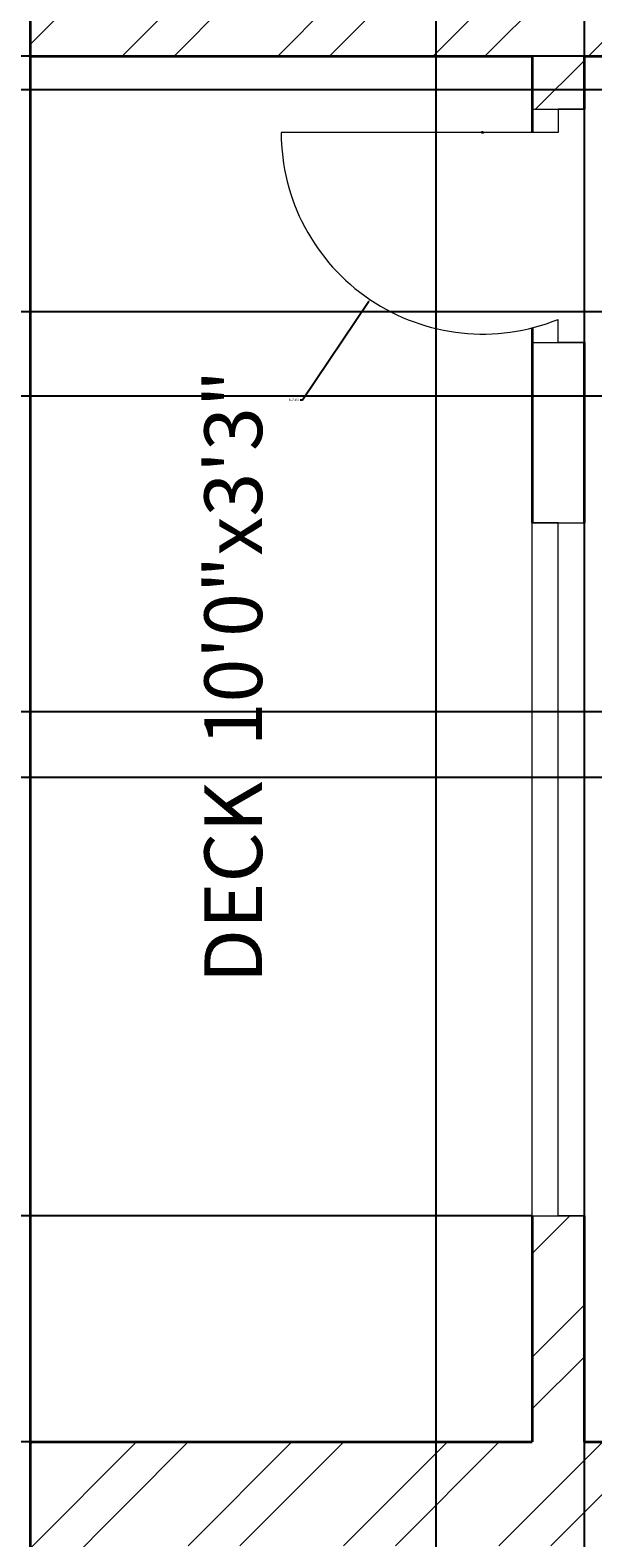
# Model space of a CAD drawing. Units: inches. Extents: x 1748 to 2382, y 1346 to 2284.
# Tile 18 of 26: x 1822 to 1871, y 1971 to 2102. Entities that reach past the tile are written whole.
import ezdxf

# ---------------------------------------------------------------- set-up
doc = ezdxf.new("R2010")
doc.units = ezdxf.units.IN
for name, color, linetype, lineweight in [('A-ANNO-DIMS', 2, 'Continuous', 18), ('A-AREA-IDEN', 7, 'Continuous', 18), ('A-DOOR', 21, 'Continuous', 18), ('A-GLAZ', 191, 'Continuous', 18), ('A-WALL', 7, 'Continuous', 35), ('A-WALL-PATT', 9, 'Continuous', 13)]:
    doc.layers.add(name, color=color, linetype=linetype, lineweight=lineweight)
doc.styles.get("Standard").update_dxf_attribs({"font": 'arial.ttf'})
doc.dimstyles.get("Standard").update_dxf_attribs({"dimtxt": 0.18, "dimasz": 0.18, "dimexe": 0.18, "dimexo": 0.0625, "dimgap": 0.09, "dimtad": 0, "dimtih": 1, "dimtoh": 1, "dimdec": 4, "dimzin": 0, "dimdsep": 46, "dimtxsty": 'Standard', "dimcen": 0.09, "dimadec": 0, "dimazin": 0, "dimtfac": 1, "dimtdec": 4, "dimtofl": 0, "dimtmove": 0, "dimatfit": 3, "dimfxl": 1, "dimtolj": 1, "dimtzin": 0, "dimarcsym": 0})

# ---------------------------------------------------------------- blocks, each defined once
blk = doc.blocks.new('WIN-60-SHALLOW')
for p, q in [((0, 60), (4.5, 60)), ((0, 60), (0, 0)), ((4.5, 60), (2.25, 60)), ((2.25, 60), (2.25, 0)), ((4.5, 60), (4.5, 0)), ((2.25, 0), (0, 0)), ((0, 0), (4.5, 0))]:
    blk.add_line(p, q)
blk = doc.blocks.new('*D41')
at = {"layer": 'A-ANNO-DIMS', "color": 0, "lineweight": -2, "transparency": 16777216}
for p, q in [((1821.96, 1854.91), (1821.96, 2274.93)), ((1822.14, 2274.75), (1839.16, 2274.75)), ((1856.96, 2274.75), (1839.95, 2274.75)), ((1857.14, 1854.91), (1857.14, 2274.93))]:
    blk.add_line(p, q, dxfattribs=at)
at = {"layer": 'A-ANNO-DIMS', "color": 0, "transparency": 16777216}
for points in [[(1822.14, 2274.78), (1822.14, 2274.72), (1821.96, 2274.75)], [(1856.96, 2274.78), (1856.96, 2274.72), (1857.14, 2274.75)]]:
    blk.add_solid(points, dxfattribs=at)
at = {"layer": 'Defpoints', "color": 0, "transparency": 16777216}
for p in [(1857.14, 2274.75), (1821.96, 1854.85), (1857.14, 1854.85)]:
    blk.add_point(p, dxfattribs=at)
at = {"layer": 'A-ANNO-DIMS', "color": 0, "transparency": 16777216, "insert": (1839.55, 2274.75), "char_height": 0.18, "attachment_point": 5}
blk.add_mtext('\\A1;35.18', dxfattribs=at)
blk = doc.blocks.new('*D45')
at = {"layer": 'A-ANNO-DIMS', "color": 0, "lineweight": -2, "transparency": 16777216}
for p, q in [((1821.9, 2232.85), (1779.88, 2232.85)), ((1780.06, 2232.67), (1780.06, 2116.07)), ((1780.06, 1999.11), (1780.06, 2115.71)), ((1865.4, 1998.93), (1779.88, 1998.93))]:
    blk.add_line(p, q, dxfattribs=at)
at = {"layer": 'A-ANNO-DIMS', "color": 0, "transparency": 16777216}
for points in [[(1780.03, 2232.67), (1780.09, 2232.67), (1780.06, 2232.85)], [(1780.03, 1999.11), (1780.09, 1999.11), (1780.06, 1998.93)]]:
    blk.add_solid(points, dxfattribs=at)
at = {"layer": 'Defpoints', "color": 0, "transparency": 16777216}
for p in [(1780.06, 2232.85), (1821.96, 2232.85), (1865.46, 1998.93)]:
    blk.add_point(p, dxfattribs=at)
at = {"layer": 'A-ANNO-DIMS', "color": 0, "transparency": 16777216, "insert": (1780.06, 2115.89), "char_height": 0.18, "attachment_point": 5}
blk.add_mtext('\\A1;233.9', dxfattribs=at)
blk = doc.blocks.new('*D50')
at = {"layer": 'A-ANNO-DIMS', "color": 0, "lineweight": -2, "transparency": 16777216}
for p, q in [((1869.96, 2223.79), (1869.96, 1360.47)), ((1908.44, 2223.79), (1908.44, 1360.47)), ((1870.14, 1360.65), (1888.81, 1360.65)), ((1908.26, 1360.65), (1889.6, 1360.65))]:
    blk.add_line(p, q, dxfattribs=at)
at = {"layer": 'A-ANNO-DIMS', "color": 0, "transparency": 16777216}
for points in [[(1870.14, 1360.68), (1870.14, 1360.62), (1869.96, 1360.65)], [(1908.26, 1360.68), (1908.26, 1360.62), (1908.44, 1360.65)]]:
    blk.add_solid(points, dxfattribs=at)
at = {"layer": 'Defpoints', "color": 0, "transparency": 16777216}
for p in [(1869.96, 2223.85), (1908.44, 2223.85), (1908.44, 1360.65)]:
    blk.add_point(p, dxfattribs=at)
at = {"layer": 'A-ANNO-DIMS', "color": 0, "transparency": 16777216, "insert": (1889.2, 1360.65), "char_height": 0.18, "attachment_point": 5}
blk.add_mtext('\\A1;38.48', dxfattribs=at)
blk = doc.blocks.new('*D57')
at = {"layer": 'A-ANNO-DIMS', "color": 0, "lineweight": -2, "transparency": 16777216}
for p, q in [((2288.4, 2099.35), (1779.88, 2099.35)), ((1780.06, 2099.17), (1780.06, 2088.46)), ((1780.06, 2077.38), (1780.06, 2088.09)), ((2288.4, 2077.2), (1779.88, 2077.2))]:
    blk.add_line(p, q, dxfattribs=at)
at = {"layer": 'A-ANNO-DIMS', "color": 0, "transparency": 16777216}
for points in [[(1780.03, 2099.17), (1780.09, 2099.17), (1780.06, 2099.35)], [(1780.03, 2077.38), (1780.09, 2077.38), (1780.06, 2077.2)]]:
    blk.add_solid(points, dxfattribs=at)
at = {"layer": 'Defpoints', "color": 0, "transparency": 16777216}
for p in [(1780.06, 2099.35), (2288.46, 2099.35), (2288.46, 2077.2)]:
    blk.add_point(p, dxfattribs=at)
at = {"layer": 'A-ANNO-DIMS', "color": 0, "transparency": 16777216, "insert": (1780.06, 2088.28), "char_height": 0.18, "attachment_point": 5}
blk.add_mtext('\\A1;22.15', dxfattribs=at)
blk = doc.blocks.new('*D63')
at = {"layer": 'A-ANNO-DIMS', "color": 0, "lineweight": -2, "transparency": 16777216}
for p, q in [((2253.72, 2042.57), (1779.88, 2042.57)), ((1780.06, 2042.39), (1780.06, 2039.92)), ((1780.06, 2037.08), (1780.06, 2039.55)), ((2253.72, 2036.9), (1779.88, 2036.9))]:
    blk.add_line(p, q, dxfattribs=at)
at = {"layer": 'A-ANNO-DIMS', "color": 0, "transparency": 16777216}
for points in [[(1780.03, 2042.39), (1780.09, 2042.39), (1780.06, 2042.57)], [(1780.03, 2037.08), (1780.09, 2037.08), (1780.06, 2036.9)]]:
    blk.add_solid(points, dxfattribs=at)
at = {"layer": 'Defpoints', "color": 0, "transparency": 16777216}
for p in [(1780.06, 2042.57), (2253.78, 2042.57), (2253.78, 2036.9)]:
    blk.add_point(p, dxfattribs=at)
at = {"layer": 'A-ANNO-DIMS', "color": 0, "transparency": 16777216, "insert": (1780.06, 2039.74), "char_height": 0.18, "attachment_point": 5}
blk.add_mtext('\\A1;5.673', dxfattribs=at)
blk = doc.blocks.new('*D69')
at = {"layer": 'A-ANNO-DIMS', "color": 0, "lineweight": -2, "transparency": 16777216}
for p, q in [((1865.4, 1998.93), (1779.88, 1998.93)), ((1780.06, 1998.75), (1780.06, 1989.32)), ((1780.06, 1979.53), (1780.06, 1988.96)), ((1821.9, 1979.35), (1779.88, 1979.35))]:
    blk.add_line(p, q, dxfattribs=at)
at = {"layer": 'A-ANNO-DIMS', "color": 0, "transparency": 16777216}
for points in [[(1780.03, 1998.75), (1780.09, 1998.75), (1780.06, 1998.93)], [(1780.03, 1979.53), (1780.09, 1979.53), (1780.06, 1979.35)]]:
    blk.add_solid(points, dxfattribs=at)
at = {"layer": 'Defpoints', "color": 0, "transparency": 16777216}
for p in [(1780.06, 1998.93), (1865.46, 1998.93), (1821.96, 1979.35)]:
    blk.add_point(p, dxfattribs=at)
at = {"layer": 'A-ANNO-DIMS', "color": 0, "transparency": 16777216, "insert": (1780.06, 1989.14), "char_height": 0.18, "attachment_point": 5}
blk.add_mtext('\\A1;19.58', dxfattribs=at)
blk = doc.blocks.new('*D76')
at = {"layer": 'A-ANNO-DIMS', "color": 0, "lineweight": -2, "transparency": 16777216}
for p, q in [((2025.9, 2096.43), (1779.88, 2096.43)), ((1780.06, 2096.25), (1780.06, 2083.35)), ((1780.06, 2070.08), (1780.06, 2082.98)), ((2025.9, 2069.9), (1779.88, 2069.9))]:
    blk.add_line(p, q, dxfattribs=at)
at = {"layer": 'A-ANNO-DIMS', "color": 0, "transparency": 16777216}
for points in [[(1780.03, 2096.25), (1780.09, 2096.25), (1780.06, 2096.43)], [(1780.03, 2070.08), (1780.09, 2070.08), (1780.06, 2069.9)]]:
    blk.add_solid(points, dxfattribs=at)
at = {"layer": 'Defpoints', "color": 0, "transparency": 16777216}
for p in [(1780.06, 2096.43), (2025.96, 2096.43), (2025.96, 2069.9)]:
    blk.add_point(p, dxfattribs=at)
at = {"layer": 'A-ANNO-DIMS', "color": 0, "transparency": 16777216, "insert": (1780.06, 2083.16), "char_height": 0.18, "attachment_point": 5}
blk.add_mtext('\\A1;26.535', dxfattribs=at)
blk = doc.blocks.new('*D94')
at = {"layer": 'A-ANNO-DIMS', "color": 0, "lineweight": -2, "transparency": 16777216}
for p, q in [((1861.17, 2092.66), (1861.17, 2092.84)), ((1861.08, 2092.75), (1861.26, 2092.75)), ((1845.55, 2069.59), (1851.31, 2078.13)), ((1845.37, 2069.59), (1845.55, 2069.59))]:
    blk.add_line(p, q, dxfattribs=at)
at = {"layer": 'A-ANNO-DIMS', "color": 0, "transparency": 16777216}
blk.add_solid([(1851.28, 2078.14), (1851.33, 2078.11), (1851.41, 2078.27)], dxfattribs=at)
at = {"layer": 'Defpoints', "color": 0, "transparency": 16777216}
for p in [(1861.17, 2092.75), (1851.41, 2078.27)]:
    blk.add_point(p, dxfattribs=at)
at = {"layer": 'A-ANNO-DIMS', "color": 0, "transparency": 16777216, "insert": (1844.82, 2069.59), "char_height": 0.18, "attachment_point": 5}
blk.add_mtext('\\A1;R17.464', dxfattribs=at)

msp = doc.modelspace()

# ---------------------------------------------------------------- hatches: boundary and pattern name
at = {"layer": 'A-WALL-PATT'}
h = msp.add_hatch(dxfattribs=at)
h.set_pattern_fill('ANSI32', color=256)
h.paths.add_polyline_path([(1908.4445, 2232.8497), (1821.9607, 2232.8497), (1821.9607, 2223.8497), (1865.4607, 2223.8497), (1865.4607, 2209.9185), (1869.9607, 2209.9185), (1869.9607, 2223.8497), (1908.4445, 2223.8497), (1908.4445, 2228.3497)])
h.paths.add_polyline_path([(2040.0683, 2232.8497), (1968.4445, 2232.8497), (1968.4445, 2223.8497), (2025.9607, 2223.8497), (2025.9607, 2130.3497), (2032.1341, 2130.3497), (2032.1341, 2132.5997), (2032.1341, 2134.8497), (2030.4607, 2134.8497), (2030.4607, 2223.8497), (2040.0683, 2223.8497)])
h.paths.add_polyline_path([(2091.3969, 2232.8497), (2064.0683, 2232.8497), (2064.0683, 2223.8497), (2078.4607, 2223.8497), (2078.4607, 2134.8497), (2051.1563, 2134.8497), (2051.1563, 2130.3497), (2078.4607, 2130.3497), (2078.4607, 2128.6813), (2082.9607, 2128.6813), (2082.9607, 2130.3497), (2086.1879, 2130.3497), (2086.1879, 2132.5997), (2086.1879, 2134.8497), (2082.9607, 2134.8497), (2082.9607, 2223.8497), (2091.3969, 2223.8497), (2091.3969, 2228.3497)])
h.paths.add_polyline_path([(2167.0164, 2232.8497), (2115.3969, 2232.8497), (2115.3969, 2223.8497), (2130.9607, 2223.8497), (2130.9607, 2134.8497), (2106.9607, 2134.8497), (2106.9607, 2130.3497), (2135.4607, 2130.3497), (2135.4607, 2223.8497), (2167.0164, 2223.8497), (2167.0164, 2228.3497)])
h.paths.add_polyline_path([(1869.9607, 2149.9185), (1865.4607, 2149.9185), (1865.4607, 2127.8942), (1869.9607, 2127.8942)])
h.paths.add_polyline_path([(2082.9607, 2104.4871), (2080.7107, 2104.4871), (2078.4607, 2104.4871), (2078.4607, 2103.8497), (1869.9607, 2103.8497), (1869.9607, 2108.6062), (1867.7107, 2108.6062), (1865.4607, 2108.6062), (1865.4607, 2103.8497), (1821.9607, 2103.8497), (1821.9607, 2099.3497), (1865.4607, 2099.3497), (1865.4607, 2094.7509), (1869.9607, 2094.7509), (1869.9607, 2099.3497), (2025.9607, 2099.3497), (2025.9607, 2096.4326), (2030.4607, 2096.4326), (2030.4607, 2099.3497), (2082.9607, 2099.3497)])
h.paths.add_polyline_path([(1928.9457, 1401.1212), (2176.8693, 1401.1212), (2176.8693, 1438.214), (1928.9457, 1438.214)], flags=9)
h.paths.add_polyline_path([(2122.2668, 2048.1927), (2177.9387, 2048.1927), (2177.9387, 2066.85), (2122.2668, 2066.85)], flags=9)
h.paths.add_polyline_path([(2272.688, 2153.8197), (2272.688, 2216.746), (2262.3845, 2216.746), (2262.3845, 2153.8197)], flags=9)
h.paths.add_polyline_path([(2157.2928, 2166.5593), (2196.3822, 2166.5593), (2196.3822, 2185.2167), (2157.2928, 2185.2167)], flags=9)
h.paths.add_polyline_path([(2089.3407, 2162.0698), (2124.3987, 2162.0698), (2124.3987, 2180.7272), (2089.3407, 2180.7272)], flags=9)
h.paths.add_polyline_path([(2037.4521, 2160.0913), (2072.5101, 2160.0913), (2072.5101, 2178.7486), (2037.4521, 2178.7486)], flags=9)
h.paths.add_polyline_path([(1884.7894, 2104.1554), (1923.6297, 2104.1554), (1923.6297, 2122.8127), (1884.7894, 2122.8127)], flags=9)
h.paths.add_polyline_path([(1851.2832, 2142.9749), (1851.2832, 2199.3051), (1840.9796, 2199.3051), (1840.9796, 2142.9749)], flags=9)
h.paths.add_polyline_path([(1844.8763, 2017.2834), (1844.8763, 2073.6136), (1834.5728, 2073.6136), (1834.5728, 2017.2834)], flags=9)
h.paths.add_polyline_path([(1897.1577, 2073.1279), (1935.9981, 2073.1279), (1935.9981, 2091.7853), (1897.1577, 2091.7853)], flags=9)
h.paths.add_polyline_path([(1952.3395, 1802.4231), (2008.0114, 1802.4231), (2008.0114, 1821.0805), (1952.3395, 1821.0805)], flags=9)
h.paths.add_polyline_path([(1978.8184, 1857.6841), (2017.7338, 1857.6841), (2017.7338, 1876.3415), (1978.8184, 1876.3415)], flags=9)
h.paths.add_polyline_path([(1979.6513, 1925.9516), (2008.8089, 1925.9516), (2008.8089, 1944.6089), (1979.6513, 1944.6089)], flags=9)
h.paths.add_polyline_path([(1838.5553, 1860.3527), (1877.3957, 1860.3527), (1877.3957, 1879.01), (1838.5553, 1879.01)], flags=9)
h.paths.add_polyline_path([(1883.9018, 1787.3013), (1883.9018, 1843.6315), (1873.5983, 1843.6315), (1873.5983, 1787.3013)], flags=9)
h.paths.add_polyline_path([(1873.7079, 1509.1938), (1873.7079, 1583.7709), (1863.4044, 1583.7709), (1863.4044, 1509.1938)], flags=9)
h.paths.add_polyline_path([(1916.2259, 1603.3681), (1955.0663, 1603.3681), (1955.0663, 1622.0254), (1916.2259, 1622.0254)], flags=9)
h.paths.add_polyline_path([(1876.3013, 1636.757), (1876.3013, 1693.0871), (1865.9978, 1693.0871), (1865.9978, 1636.757)], flags=9)
h.paths.add_polyline_path([(1921.3138, 1521.8316), (1964.0662, 1521.8316), (1964.0662, 1540.489), (1921.3138, 1540.489)], flags=9)
h.paths.add_polyline_path([(2017.5657, 1497.5078), (2046.7983, 1497.5078), (2046.7983, 1516.1651), (2017.5657, 1516.1651)], flags=9)
h.paths.add_polyline_path([(2066.8661, 1499.3902), (2096.0988, 1499.3902), (2096.0988, 1518.0475), (2066.8661, 1518.0475)], flags=9)
h.paths.add_polyline_path([(2155.4835, 1571.6596), (2198.2358, 1571.6596), (2198.2358, 1590.3169), (2155.4835, 1590.3169)], flags=9)
h.paths.add_polyline_path([(2094.9136, 1664.6812), (2150.5855, 1664.6812), (2150.5855, 1683.3386), (2094.9136, 1683.3386)], flags=9)
h.paths.add_polyline_path([(2257.6902, 1863.1628), (2269.8935, 1863.1628), (2269.8935, 1873.4664), (2257.6902, 1873.4664)], flags=9)
h.paths.add_polyline_path([(2164.0748, 1880.3089), (2189.8694, 1880.3089), (2189.8694, 1890.6124), (2164.0748, 1890.6124)], flags=9)
h.paths.add_polyline_path([(2239.4394, 1931.0585), (2268.8187, 1931.0585), (2268.8187, 1949.7159), (2239.4394, 1949.7159)], flags=9)
h = msp.add_hatch(dxfattribs=at)
h.set_pattern_fill('ANSI32', color=256)
h.paths.add_polyline_path([(2297.4607, 2232.8497), (2203.0164, 2232.8497), (2203.0164, 2223.8497), (2244.9607, 2223.8497), (2244.9607, 2127.8554), (2249.4607, 2127.8554), (2249.4607, 2223.8497), (2297.4607, 2223.8497)])
h.paths.add_polyline_path([(2297.4607, 2103.8497), (2249.4607, 2103.8497), (2249.4607, 2106.7497), (2247.2107, 2106.7497), (2244.9607, 2106.7497), (2244.9607, 2103.8497), (2130.9607, 2103.8497), (2130.9607, 2099.3497), (2288.4607, 2099.3497), (2288.4607, 2077.2008), (2297.4607, 2077.2008)])
h.paths.add_polyline_path([(1928.9457, 1401.1212), (2176.8693, 1401.1212), (2176.8693, 1438.214), (1928.9457, 1438.214)], flags=9)
h.paths.add_polyline_path([(2122.2668, 2048.1927), (2177.9387, 2048.1927), (2177.9387, 2066.85), (2122.2668, 2066.85)], flags=9)
h.paths.add_polyline_path([(2272.688, 2153.8197), (2272.688, 2216.746), (2262.3845, 2216.746), (2262.3845, 2153.8197)], flags=25)
h.paths.add_polyline_path([(2157.2928, 2166.5593), (2196.3822, 2166.5593), (2196.3822, 2185.2167), (2157.2928, 2185.2167)], flags=9)
h.paths.add_polyline_path([(2089.3407, 2162.0698), (2124.3987, 2162.0698), (2124.3987, 2180.7272), (2089.3407, 2180.7272)], flags=9)
h.paths.add_polyline_path([(2037.4521, 2160.0913), (2072.5101, 2160.0913), (2072.5101, 2178.7486), (2037.4521, 2178.7486)], flags=9)
h.paths.add_polyline_path([(1884.7894, 2104.1554), (1923.6297, 2104.1554), (1923.6297, 2122.8127), (1884.7894, 2122.8127)], flags=9)
h.paths.add_polyline_path([(1851.2832, 2142.9749), (1851.2832, 2199.3051), (1840.9796, 2199.3051), (1840.9796, 2142.9749)], flags=9)
h.paths.add_polyline_path([(1844.8763, 2017.2834), (1844.8763, 2073.6136), (1834.5728, 2073.6136), (1834.5728, 2017.2834)], flags=9)
h.paths.add_polyline_path([(1897.1577, 2073.1279), (1935.9981, 2073.1279), (1935.9981, 2091.7853), (1897.1577, 2091.7853)], flags=9)
h.paths.add_polyline_path([(1952.3395, 1802.4231), (2008.0114, 1802.4231), (2008.0114, 1821.0805), (1952.3395, 1821.0805)], flags=9)
h.paths.add_polyline_path([(1978.8184, 1857.6841), (2017.7338, 1857.6841), (2017.7338, 1876.3415), (1978.8184, 1876.3415)], flags=9)
h.paths.add_polyline_path([(1979.6513, 1925.9516), (2008.8089, 1925.9516), (2008.8089, 1944.6089), (1979.6513, 1944.6089)], flags=9)
h.paths.add_polyline_path([(1838.5553, 1860.3527), (1877.3957, 1860.3527), (1877.3957, 1879.01), (1838.5553, 1879.01)], flags=9)
h.paths.add_polyline_path([(1883.9018, 1787.3013), (1883.9018, 1843.6315), (1873.5983, 1843.6315), (1873.5983, 1787.3013)], flags=9)
h.paths.add_polyline_path([(1873.7079, 1509.1938), (1873.7079, 1583.7709), (1863.4044, 1583.7709), (1863.4044, 1509.1938)], flags=9)
h.paths.add_polyline_path([(1916.2259, 1603.3681), (1955.0663, 1603.3681), (1955.0663, 1622.0254), (1916.2259, 1622.0254)], flags=9)
h.paths.add_polyline_path([(1876.3013, 1636.757), (1876.3013, 1693.0871), (1865.9978, 1693.0871), (1865.9978, 1636.757)], flags=9)
h.paths.add_polyline_path([(1921.3138, 1521.8316), (1964.0662, 1521.8316), (1964.0662, 1540.489), (1921.3138, 1540.489)], flags=9)
h.paths.add_polyline_path([(2017.5657, 1497.5078), (2046.7983, 1497.5078), (2046.7983, 1516.1651), (2017.5657, 1516.1651)], flags=9)
h.paths.add_polyline_path([(2066.8661, 1499.3902), (2096.0988, 1499.3902), (2096.0988, 1518.0475), (2066.8661, 1518.0475)], flags=9)
h.paths.add_polyline_path([(2155.4835, 1571.6596), (2198.2358, 1571.6596), (2198.2358, 1590.3169), (2155.4835, 1590.3169)], flags=9)
h.paths.add_polyline_path([(2094.9136, 1664.6812), (2150.5855, 1664.6812), (2150.5855, 1683.3386), (2094.9136, 1683.3386)], flags=9)
h.paths.add_polyline_path([(2257.6902, 1863.1628), (2269.8935, 1863.1628), (2269.8935, 1873.4664), (2257.6902, 1873.4664)], flags=9)
h.paths.add_polyline_path([(2164.0748, 1880.3089), (2189.8694, 1880.3089), (2189.8694, 1890.6124), (2164.0748, 1890.6124)], flags=9)
h.paths.add_polyline_path([(2239.4394, 1931.0585), (2268.8187, 1931.0585), (2268.8187, 1949.7159), (2239.4394, 1949.7159)], flags=9)
h = msp.add_hatch(dxfattribs=at)
h.set_pattern_fill('ANSI32', color=256)
h.paths.add_polyline_path([(1919.6777, 1476.8497), (1900.6426, 1476.8497), (1900.6426, 1522.0826), (1898.3926, 1522.0826), (1896.1426, 1522.0826), (1896.1426, 1476.8497), (1857.1426, 1476.8497), (1857.1426, 1467.8497), (1896.1426, 1467.8497), (1919.6777, 1467.8497), (1919.6777, 1472.3497)])
h.paths.add_polyline_path([(2018.7873, 1472.3497), (2018.7873, 1476.8497), (2010.9607, 1476.8497), (2010.9607, 1560.8497), (2034.9607, 1560.8497), (2034.9607, 1565.3497), (2006.4607, 1565.3497), (2006.4607, 1476.8497), (1955.6777, 1476.8497), (1955.6777, 1467.8497), (2018.7873, 1467.8497)])
h.paths.add_polyline_path([(2152.3354, 1472.3497), (2152.3354, 1476.8497), (2115.9607, 1476.8497), (2115.9607, 1565.3497), (2109.2204, 1565.3497), (2109.2204, 1563.0997), (2109.2204, 1560.8497), (2111.4607, 1560.8497), (2111.4607, 1476.8497), (2095.3617, 1476.8497), (2095.3617, 1467.8497), (2152.3354, 1467.8497)])
h.paths.add_polyline_path([(2071.3617, 1476.8497), (2063.4607, 1476.8497), (2063.4607, 1560.8497), (2090.1865, 1560.8497), (2090.1865, 1565.3497), (2063.4607, 1565.3497), (2063.4607, 1572.5485), (2061.2107, 1572.5485), (2058.9607, 1572.5485), (2058.9607, 1565.3497), (2055.6281, 1565.3497), (2055.6281, 1560.8497), (2058.9607, 1560.8497), (2058.9607, 1476.8497), (2042.7873, 1476.8497), (2042.7873, 1467.8497), (2071.3617, 1467.8497), (2071.3617, 1472.3497)])
h.paths.add_polyline_path([(2297.4607, 1506.5652), (2288.4607, 1506.5652), (2288.4607, 1476.8497), (2212.3354, 1476.8497), (2212.3354, 1467.8497), (2297.4607, 1467.8497)])
h.paths.add_polyline_path([(2297.4607, 1645.3038), (2288.4607, 1645.3038), (2288.4607, 1605.8497), (2058.9607, 1605.8497), (2058.9607, 1600.1857), (2061.2107, 1600.1857), (2063.4607, 1600.1857), (2063.4607, 1601.3497), (2288.4607, 1601.3497), (2288.4607, 1566.5652), (2297.4607, 1566.5652)])
h.paths.add_polyline_path([(2010.9607, 1609.0561), (2008.7107, 1609.0561), (2006.4607, 1609.0561), (2006.4607, 1605.8497), (1900.6426, 1605.8497), (1900.6426, 1609.7171), (1898.3926, 1609.7171), (1896.1426, 1609.7171), (1896.1426, 1605.8497), (1857.1426, 1605.8497), (1857.1426, 1601.3497), (1896.1426, 1601.3497), (1896.1426, 1542.5447), (1900.6426, 1542.5447), (1900.6426, 1601.3497), (2010.9607, 1601.3497)])
h.paths.add_polyline_path([(1928.9457, 1401.1212), (2176.8693, 1401.1212), (2176.8693, 1438.214), (1928.9457, 1438.214)], flags=9)
h.paths.add_polyline_path([(2122.2668, 2048.1927), (2177.9387, 2048.1927), (2177.9387, 2066.85), (2122.2668, 2066.85)], flags=9)
h.paths.add_polyline_path([(2272.688, 2153.8197), (2272.688, 2216.746), (2262.3845, 2216.746), (2262.3845, 2153.8197)], flags=9)
h.paths.add_polyline_path([(2157.2928, 2166.5593), (2196.3822, 2166.5593), (2196.3822, 2185.2167), (2157.2928, 2185.2167)], flags=9)
h.paths.add_polyline_path([(2089.3407, 2162.0698), (2124.3987, 2162.0698), (2124.3987, 2180.7272), (2089.3407, 2180.7272)], flags=9)
h.paths.add_polyline_path([(2037.4521, 2160.0913), (2072.5101, 2160.0913), (2072.5101, 2178.7486), (2037.4521, 2178.7486)], flags=9)
h.paths.add_polyline_path([(1884.7894, 2104.1554), (1923.6297, 2104.1554), (1923.6297, 2122.8127), (1884.7894, 2122.8127)], flags=9)
h.paths.add_polyline_path([(1851.2832, 2142.9749), (1851.2832, 2199.3051), (1840.9796, 2199.3051), (1840.9796, 2142.9749)], flags=9)
h.paths.add_polyline_path([(1844.8763, 2017.2834), (1844.8763, 2073.6136), (1834.5728, 2073.6136), (1834.5728, 2017.2834)], flags=9)
h.paths.add_polyline_path([(1897.1577, 2073.1279), (1935.9981, 2073.1279), (1935.9981, 2091.7853), (1897.1577, 2091.7853)], flags=9)
h.paths.add_polyline_path([(1952.3395, 1802.4231), (2008.0114, 1802.4231), (2008.0114, 1821.0805), (1952.3395, 1821.0805)], flags=9)
h.paths.add_polyline_path([(1978.8184, 1857.6841), (2017.7338, 1857.6841), (2017.7338, 1876.3415), (1978.8184, 1876.3415)], flags=9)
h.paths.add_polyline_path([(1979.6513, 1925.9516), (2008.8089, 1925.9516), (2008.8089, 1944.6089), (1979.6513, 1944.6089)], flags=9)
h.paths.add_polyline_path([(1838.5553, 1860.3527), (1877.3957, 1860.3527), (1877.3957, 1879.01), (1838.5553, 1879.01)], flags=9)
h.paths.add_polyline_path([(1883.9018, 1787.3013), (1883.9018, 1843.6315), (1873.5983, 1843.6315), (1873.5983, 1787.3013)], flags=9)
h.paths.add_polyline_path([(1873.7079, 1509.1938), (1873.7079, 1583.7709), (1863.4044, 1583.7709), (1863.4044, 1509.1938)], flags=9)
h.paths.add_polyline_path([(1916.2259, 1603.3681), (1955.0663, 1603.3681), (1955.0663, 1622.0254), (1916.2259, 1622.0254)], flags=9)
h.paths.add_polyline_path([(1876.3013, 1636.757), (1876.3013, 1693.0871), (1865.9978, 1693.0871), (1865.9978, 1636.757)], flags=9)
h.paths.add_polyline_path([(1921.3138, 1521.8316), (1964.0662, 1521.8316), (1964.0662, 1540.489), (1921.3138, 1540.489)], flags=9)
h.paths.add_polyline_path([(2017.5657, 1497.5078), (2046.7983, 1497.5078), (2046.7983, 1516.1651), (2017.5657, 1516.1651)], flags=9)
h.paths.add_polyline_path([(2066.8661, 1499.3902), (2096.0988, 1499.3902), (2096.0988, 1518.0475), (2066.8661, 1518.0475)], flags=9)
h.paths.add_polyline_path([(2155.4835, 1571.6596), (2198.2358, 1571.6596), (2198.2358, 1590.3169), (2155.4835, 1590.3169)], flags=25)
h.paths.add_polyline_path([(2094.9136, 1664.6812), (2150.5855, 1664.6812), (2150.5855, 1683.3386), (2094.9136, 1683.3386)], flags=9)
h.paths.add_polyline_path([(2257.6902, 1863.1628), (2269.8935, 1863.1628), (2269.8935, 1873.4664), (2257.6902, 1873.4664)], flags=9)
h.paths.add_polyline_path([(2164.0748, 1880.3089), (2189.8694, 1880.3089), (2189.8694, 1890.6124), (2164.0748, 1890.6124)], flags=9)
h.paths.add_polyline_path([(2239.4394, 1931.0585), (2268.8187, 1931.0585), (2268.8187, 1949.7159), (2239.4394, 1949.7159)], flags=9)
h = msp.add_hatch(dxfattribs=at)
h.set_pattern_fill('ANSI32', color=256)
h.paths.add_polyline_path([(1900.6426, 1652.723), (1896.1426, 1652.723), (1896.1426, 1629.9029), (1900.6426, 1629.9029)])
h.paths.add_polyline_path([(2206.0699, 1859.3497), (2197.0699, 1859.3497), (2197.0699, 1734.8497), (2206.0699, 1734.8497)], flags=17)
h.paths.add_polyline_path([(2297.4607, 1865.3269), (2288.4607, 1865.3269), (2288.4607, 1734.8497), (2206.0699, 1734.8497), (2180.4551, 1734.8497), (2180.4551, 1725.8497), (2197.0699, 1725.8497), (2206.0699, 1725.8497), (2288.4607, 1725.8497), (2288.4607, 1705.3038), (2297.4607, 1705.3038)])
h.paths.add_polyline_path([(2139.9607, 1815.8001), (2135.4607, 1815.8001), (2130.9607, 1815.8001), (2130.9607, 1734.8497), (1900.6426, 1734.8497), (1900.6426, 1738.9477), (1898.3926, 1738.9477), (1896.1426, 1738.9477), (1896.1426, 1734.8497), (1857.1426, 1734.8497), (1857.1426, 1725.8497), (1896.1426, 1725.8497), (1896.1426, 1712.723), (1900.6426, 1712.723), (1900.6426, 1725.8497), (2006.4607, 1725.8497), (2006.4607, 1637.448), (2010.9607, 1637.448), (2010.9607, 1725.8497), (2139.9607, 1725.8497), (2147.389, 1725.8497), (2147.389, 1730.3497), (2147.389, 1734.8497), (2139.9607, 1734.8497)])
h.paths.add_polyline_path([(2149.8497, 1917.8497), (2149.8497, 1922.3497), (2139.9607, 1922.3497), (2139.9607, 1979.3497), (2030.4607, 1979.3497), (2030.4607, 2069.8971), (2028.2107, 2069.8971), (2025.9607, 2069.8971), (2025.9607, 1979.3497), (1869.9607, 1979.3497), (1869.9607, 1998.93), (1865.4607, 1998.93), (1865.4607, 1979.3497), (1821.9607, 1979.3497), (1821.9607, 1952.7922), (1826.9306, 1952.7922), (1830.9607, 1952.7922), (1830.9607, 1970.3497), (1962.9607, 1970.3497), (1962.9607, 1926.5713), (1967.4607, 1926.5713), (1967.4607, 1970.3497), (2027.4607, 1970.3497), (2027.4607, 1898.3497), (2004.9604, 1898.3497), (2004.9604, 1893.8497), (2027.4607, 1893.8497), (2027.4607, 1859.3497), (1958.8973, 1859.3497), (1958.8973, 1854.8497), (2047.917, 1854.8497), (2047.917, 1859.3497), (2031.9607, 1859.3497), (2031.9607, 1970.3497), (2130.9607, 1970.3497), (2130.9607, 1859.3497), (2104.9565, 1859.3497), (2104.9565, 1854.8497), (2130.9607, 1854.8497), (2130.9607, 1849.0684), (2139.9607, 1849.0684), (2139.9607, 1913.3497), (2149.8497, 1913.3497)])
h.paths.add_polyline_path([(1928.9996, 1859.3497), (1830.9607, 1859.3497), (1830.9607, 1892.7922), (1821.9607, 1892.7922), (1821.9607, 1854.8497), (1896.1426, 1854.8497), (1896.1426, 1836.6443), (1898.378, 1836.6443), (1900.6426, 1836.6443), (1900.6426, 1854.8497), (1928.9996, 1854.8497), (1928.9996, 1857.0997)])
h.paths.add_polyline_path([(1980.9604, 1896.0997), (1980.9604, 1898.3497), (1967.4607, 1898.3497), (1967.4607, 1902.3846), (1962.9607, 1902.3846), (1962.9607, 1859.3497), (1967.4607, 1859.3497), (1967.4607, 1893.8497), (1980.9604, 1893.8497)], flags=17)
h.paths.add_polyline_path([(1900.6426, 1776.6443), (1896.1426, 1776.6443), (1896.1426, 1758.0891), (1900.6426, 1758.0891)], flags=17)
h.paths.add_polyline_path([(2297.4607, 2017.2008), (2288.4607, 2017.2008), (2288.4607, 1979.3497), (2213.4607, 1979.3497), (2213.4607, 1922.3497), (2183.3516, 1922.3497), (2183.3516, 1913.3497), (2213.4607, 1913.3497), (2236.234, 1913.3497), (2236.234, 1922.3497), (2222.4607, 1922.3497), (2222.4607, 1931.3497), (2222.4607, 1970.3497), (2288.4607, 1970.3497), (2288.4607, 1922.3497), (2272.1921, 1922.3497), (2272.1921, 1913.3497), (2288.4607, 1913.3497), (2288.4607, 1901.3269), (2297.4607, 1901.3269)])

# ---------------------------------------------------------------- linework, layer by layer
at = {"layer": 'A-DOOR'}
for p, q in [((1865.4607, 2094.7509), (1869.9607, 2094.7509)), ((1869.9607, 2094.7509), (1867.7107, 2094.7509)), ((1867.7107, 2094.7509), (1867.7107, 2092.7509)), ((1867.7107, 2092.7509), (1843.7107, 2092.7509)), ((1867.7107, 2074.5562), (1867.7107, 2076.5562)), ((1865.4607, 2074.5562), (1869.9607, 2074.5562)), ((1869.9607, 2074.5562), (1867.7107, 2074.5562))]:
    msp.add_line(p, q, dxfattribs=at)
msp.add_arc((1861.1746, 2092.7509), 17.464, 180, 291.978475, dxfattribs=at)
at = {"layer": 'A-WALL'}
for p, q in [((1821.9607, 2232.8497), (1821.9607, 1952.7922)), ((1821.9607, 2099.3497), (1865.4607, 2099.3497)), ((1865.4607, 2099.3497), (1865.4607, 2092.7509)), ((1869.9607, 2099.3497), (1869.9607, 2094.7509)), ((1869.9607, 2099.3497), (2025.9607, 2099.3497)), ((1865.4607, 2075.8211), (1865.4607, 2058.93)), ((1869.9607, 2074.5562), (1869.9607, 2058.93)), ((1865.4607, 1998.93), (1865.4607, 1979.3497)), ((1869.9607, 1998.93), (1869.9607, 1979.3497)), ((1821.9607, 1979.3497), (1865.4607, 1979.3497)), ((1869.9607, 1979.3497), (2025.9607, 1979.3497))]:
    msp.add_line(p, q, dxfattribs=at)

# ---------------------------------------------------------------- block references
at = {"layer": 'A-GLAZ', "extrusion": (0, 0, -1), "zscale": -1, "rotation": 180}
msp.add_blockref('WIN-60-SHALLOW', (-1865.461, 2058.93), dxfattribs=at)

# ---------------------------------------------------------------- texts
at = {"layer": 'A-AREA-IDEN', "insert": (1837.0608, 2019.0723), "char_height": 5, "attachment_point": 1, "rotation": 90}
msp.add_mtext_dynamic_manual_height_columns('DECK  10\'0"x3\'3"', width=143.391432, gutter_width=12.5, heights=[0], dxfattribs=at)

# ---------------------------------------------------------------- dimensions: what is measured, and where the dimension line sits
at = {"layer": 'A-ANNO-DIMS'}
for base, p1, p2, picture, middle in [((1857.1426, 2274.7497), (1821.9607, 1854.8497), (1857.1426, 1854.8497), '*D41', (1839.5517, 2274.7497)), ((1908.4445, 1360.6451), (1869.9607, 2223.8497), (1908.4445, 2223.8497), '*D50', (1889.2026, 1360.6451))]:
    dim = msp.add_linear_dim(base=base, p1=p1, p2=p2, dimstyle='Standard', override={"dimdec": 2, "dimlfac": 1, "dimrnd": 0, "dimzin": 0, "dimdsep": 46, "dimlunit": 2}, dxfattribs=at)
    dim.commit()
    dim.dimension.update_dxf_attribs({"geometry": picture, "text_midpoint": middle})
for base, p1, p2, override, picture, middle in [((1780.0607, 2232.8497), (1865.4607, 1998.93), (1821.9607, 2232.8497), {"dimdec": 1, "dimlfac": 1, "dimrnd": 0, "dimzin": 0, "dimdsep": 46, "dimlunit": 2}, '*D45', (1780.0607, 2115.8898)), ((1780.0607, 2099.3497), (2288.4607, 2077.2008), (2288.4607, 2099.3497), {"dimdec": 2, "dimlfac": 1, "dimrnd": 0, "dimzin": 0, "dimdsep": 46, "dimlunit": 2}, '*D57', (1780.0607, 2088.2752)), ((1780.06066, 2096.4326), (2025.96066, 2069.89715), (2025.96066, 2096.4326), {"dimdec": 3, "dimlfac": 1, "dimrnd": 0, "dimzin": 0, "dimdsep": 46, "dimlunit": 2}, '*D76', (1780.06066, 2083.16488)), ((1780.0607, 2042.573), (2253.7809, 2036.9), (2253.7809, 2042.573), {"dimdec": 3, "dimlfac": 1, "dimrnd": 0, "dimzin": 0, "dimdsep": 46, "dimlunit": 2}, '*D63', (1780.0607, 2039.7365)), ((1780.0607, 1998.93), (1821.9607, 1979.3497), (1865.4607, 1998.93), {"dimdec": 2, "dimlfac": 1, "dimrnd": 0, "dimzin": 0, "dimdsep": 46, "dimlunit": 2}, '*D69', (1780.0607, 1989.1398))]:
    dim = msp.add_linear_dim(base=base, p1=p1, p2=p2, angle=90, dimstyle='Standard', override=override, dxfattribs=at)
    dim.commit()
    dim.dimension.update_dxf_attribs({"geometry": picture, "text_midpoint": middle})
dim = msp.add_radius_dim(center=(1861.1746, 2092.7509), mpoint=(1851.4063, 2078.2744), dimstyle='Standard', override={"dimdec": 3, "dimlfac": 1, "dimrnd": 0, "dimzin": 0, "dimdsep": 46, "dimlunit": 2}, dxfattribs=at)
dim.commit()
dim.dimension.update_dxf_attribs({"geometry": '*D94', "text_midpoint": (1844.8159, 2069.5885), "dimtype": 164})

doc.saveas('drawing.dxf')
